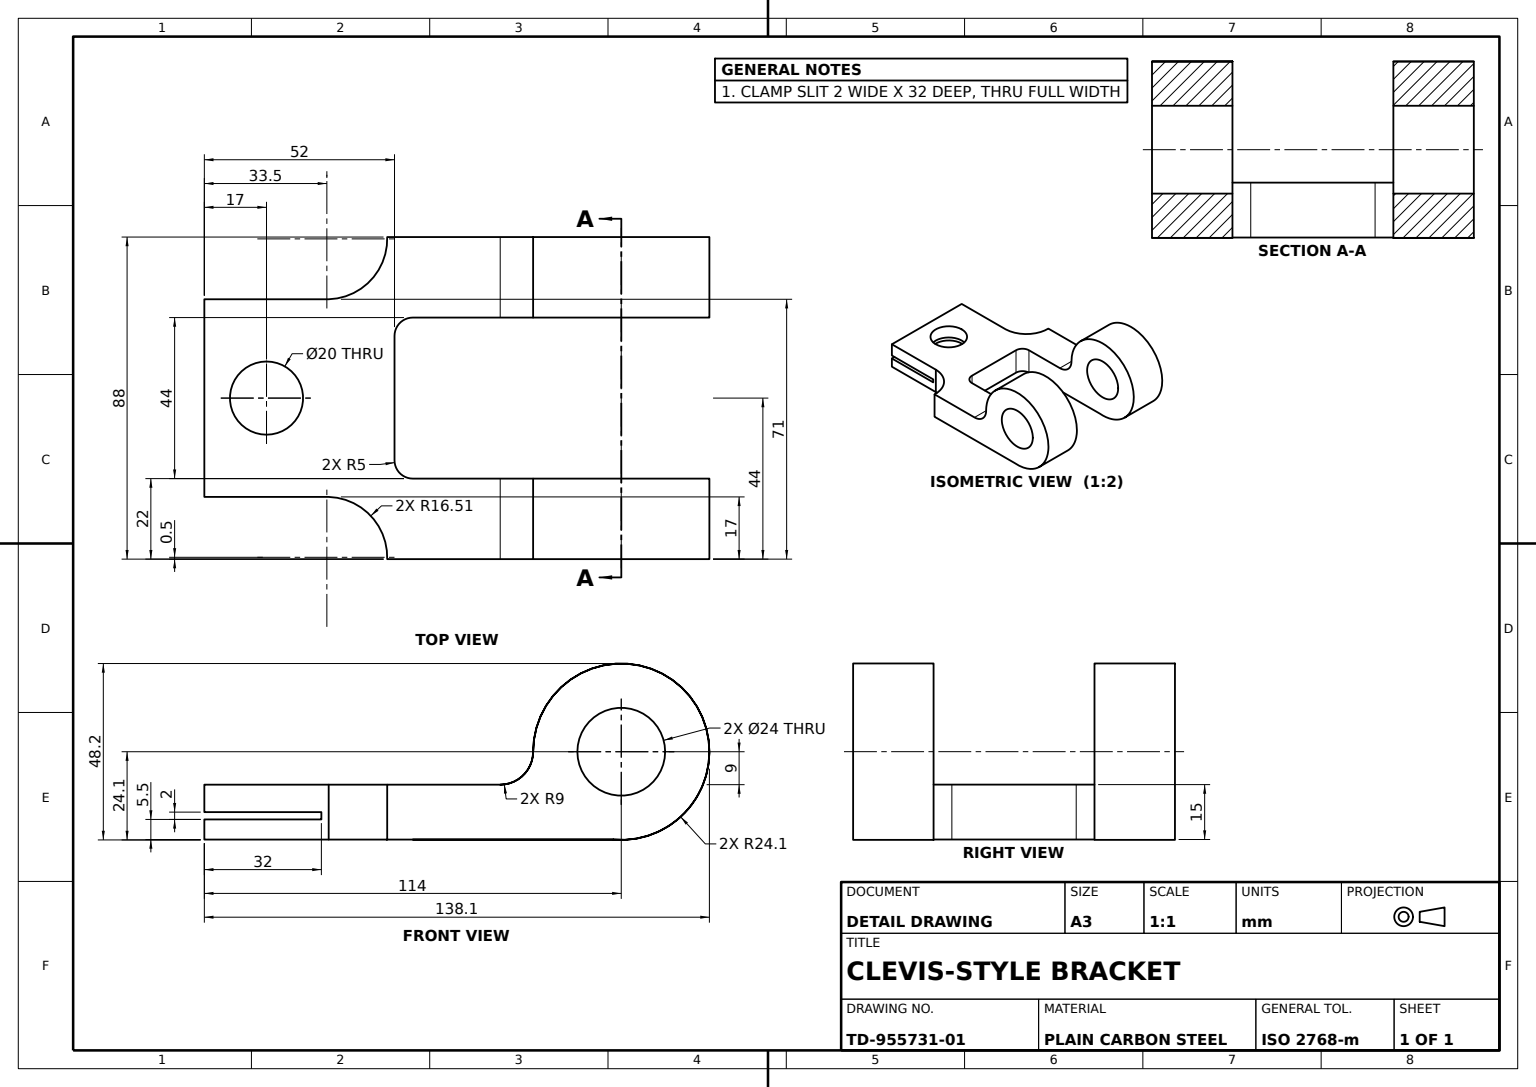
SolidWorks part; units mm, degrees
material "Plain Carbon Steel"
ref_plane "Front Plane" through (0, 0, 0) normal (0, 0, 1) x (1, 0, 0)
ref_plane "Top Plane" through (0, 0, 0) normal (0, 1, 0) x (1, 0, 0)
ref_plane "Right Plane" through (0, 0, 0) normal (1, 0, 0) x (0, 0, -1)
sketch "Base Plate Sketch" plane through (0, 0, 0) normal (0, 1, 0) x (1, 0, 0)
  line L1 (-57, -44) -> (57, -44)
  line L2 (-57, -44) -> (-57, 44)
  line L3 (-57, 44) -> (57, 44)
  line L4 (57, -44) -> (57, 44)
  line L5 (-57, -44) -> (57, 44) construction
  line L6 (-57, 44) -> (57, -44) construction
  point P0 (0, 0)
  dimension "D1" = 88
  dimension "D2" = 114
extrude "Base Plate 114x88x15" add sketch "Base Plate Sketch" along normal blind 15
sketch "Fork Eye A Sketch" plane through (0, 0, 44) normal (0, 0, 1) x (1, 0, 0)
  line L0 (-57, 15) -> (57, 15) construction
  circle A0 centre (57, 24) radius 24.1
  dimension "D1" = 48.2
  dimension "D2" = 57
  dimension "D3" = 9
extrude "Fork Eye A Ø48.2" add sketch "Fork Eye A Sketch" against normal blind 22
sketch "Fork Eye B Sketch" plane through (0, 0, -44) normal (0, 0, -1) x (-1, 0, 0)
  circle A0 centre (-57, 24) radius 24.1
  dimension "D1" = 48.2
extrude "Fork Eye B Ø48.2" add sketch "Fork Eye B Sketch" against normal blind 22
sketch "Eye Bore Sketch" plane through (0, 0, -44) normal (0, 0, -1) x (-1, 0, 0)
  circle A0 centre (-57, 24) radius 12
  dimension "D1" = 24
extrude "Eye Bore Ø24" cut sketch "Eye Bore Sketch" against normal through all
fillet "Fork Fillet R9" radius 9 2 edges at (34.6436, 15, -33) (34.6436, 15, 33)
sketch "Fork Gap Profile Sketch" plane through (0, 15, 0) normal (0, 1, 0) x (1, 0, 0)
  line L0 (-57, 44) -> (-57, -44) construction
  line L1 (-57, -44) -> (23.9, -44) construction
  line L2 (57, 22) -> (0, 22)
  line L3 (-57, 44) -> (-7, 44)
  line L4 (23.9, 44) -> (-57, 44) construction
  line L5 (-57, 27) -> (-23, 27)
  line L6 (-57, 27) -> (-57, 44)
  line L7 (-57, -44) -> (-7, -44)
  line L8 (-57, -44) -> (-57, -27)
  line L9 (-57, -27) -> (-23, -27)
  line L10 (32.9, 22) -> (81.1, 22) construction
  line L11 (-5, 17) -> (-5, -17)
  line L12 (0, -22) -> (57, -22)
  line L13 (57, -22) -> (57, 22)
  circle A0 centre (-40, 0) radius 10
  arc A1 (-23, 27) -> (-7, 44) centre (-23.5, 43.5) ccw
  arc A2 (-23, -27) -> (-7, -44) centre (-23.5, -43.5) cw
  arc A3 (-5, -17) -> (0, -22) centre (0, -17) ccw
  arc A4 (0, 22) -> (-5, 17) centre (0, 17) ccw
  point P9 (-57, 0)
  point P31 (-5, -22)
  dimension "D1" = 20
  dimension "D7" = 16.5076
  dimension "D10" = 34
  dimension "D12" = 16.5076
  dimension "D16" = 5
  dimension "D2" = 17
  dimension "D3" = 44
  dimension "D4" = 54
  dimension "D5" = 57
  dimension "D6" = 44
  dimension "D8" = 50
  dimension "D9" = 34
  dimension "D11" = 50
  dimension "D13" = 27
  dimension "D14" = 27
  dimension "D15" = 62
extrude "Fork Gap and Clamp Hole Cut" cut sketch "Fork Gap Profile Sketch" against normal through all
sketch "Clamp Slit Sketch" plane through (0, 0, -27) normal (0, 0, -1) x (-1, 0, 0)
  line L0 (57, 0) -> (57, 15) construction
  line L1 (57, 5.5) -> (25, 5.5)
  line L2 (57, 5.5) -> (57, 7.5)
  line L3 (57, 7.5) -> (25, 7.5)
  line L4 (25, 5.5) -> (25, 7.5)
  line L5 (57, 15) -> (23, 15) construction
  dimension "D1" = 2
  dimension "D2" = 7.5
  dimension "D3" = 32
extrude "Clamp Slit 2mm" cut sketch "Clamp Slit Sketch" against normal through all both and the other way through all
